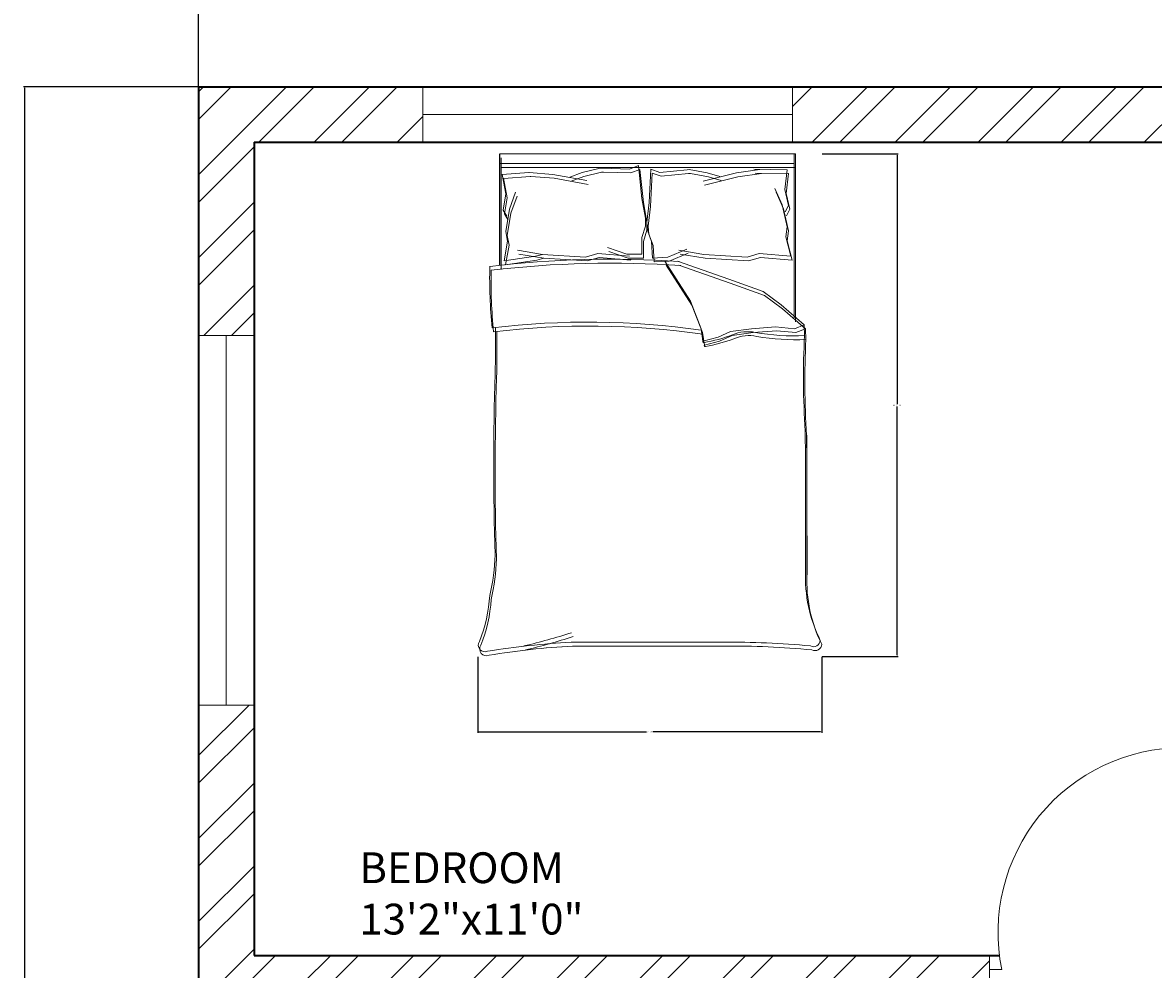
# Model space of a CAD drawing. Units: inches. Extents: x 1850 to 3445, y 1558 to 2756.
# Tile 3 of 13: x 2012 to 2195, y 2073 to 2227. Entities that reach past the tile are written whole.
import ezdxf

# ---------------------------------------------------------------- set-up
doc = ezdxf.new("R2010")
doc.units = ezdxf.units.IN
for name, color, linetype, lineweight in [('A-ANNO-DIMS', 2, 'Continuous', 18), ('A-AREA-IDEN', 7, 'Continuous', 18), ('A-DOOR', 3, 'Continuous', 18), ('A-FURN', 8, 'Continuous', 13), ('A-GLAZ', 4, 'Continuous', 18), ('A-WALL', 7, 'Continuous', 35), ('A-WALL-PATT', 252, 'Continuous', 13)]:
    doc.layers.add(name, color=color, linetype=linetype, lineweight=lineweight)
doc.styles.get("Standard").update_dxf_attribs({"font": 'arial.ttf'})
doc.dimstyles.get("Standard").update_dxf_attribs({"dimtxt": 0.18, "dimasz": 0.18, "dimexe": 0.18, "dimexo": 0.0625, "dimgap": 0.09, "dimtad": 0, "dimtih": 1, "dimtoh": 1, "dimdec": 4, "dimzin": 0, "dimdsep": 46, "dimtxsty": 'Standard', "dimcen": 0.09, "dimadec": 0, "dimazin": 0, "dimtfac": 1, "dimtdec": 4, "dimtofl": 0, "dimtmove": 0, "dimatfit": 3, "dimfxl": 1, "dimtolj": 1, "dimtzin": 0, "dimarcsym": 0})

# ---------------------------------------------------------------- blocks, each defined once
blk = doc.blocks.new('BED-PLAN')
for p, q in [((3.47, 63.33), (3.47, 81.44)), ((3.48, 63.33), (3.48, 81.44)), ((51.27, 81.44), (3.48, 81.44)), ((3.7, 62.69), (3.7, 80.8)), ((3.7, 62.69), (3.7, 80.8)), ((51.27, 81.44), (51.27, 54.83)), ((51.27, 81.44), (51.27, 54.83)), ((51.27, 81.44), (51.49, 81.44)), ((51.49, 81.44), (51.49, 80.8)), ((51.49, 80.8), (51.49, 54.19)), ((51.49, 80.8), (51.49, 54.19)), ((3.47, 79.91), (51.27, 79.91)), ((3.48, 79.91), (51.27, 79.91)), ((3.7, 79.27), (51.49, 79.27)), ((3.7, 79.27), (51.49, 79.27)), ((16.88, 78.42), (19.77, 79.14)), ((16.88, 78.42), (19.77, 79.14)), ((19.77, 79.14), (20.09, 79.14)), ((19.77, 79.14), (20.09, 79.14)), ((20.09, 79.14), (24.54, 78.99)), ((20.09, 79.14), (24.54, 78.99)), ((24.54, 78.99), (25.98, 79.57)), ((24.54, 78.99), (25.98, 79.57)), ((24.77, 78.36), (26.21, 78.93)), ((24.77, 78.36), (26.21, 78.93)), ((25.98, 79.57), (26.56, 74.22)), ((25.98, 79.57), (26.56, 74.22)), ((26.21, 78.93), (26.79, 73.58)), ((26.21, 78.93), (26.79, 73.58)), ((27.98, 78.95), (27.73, 73.58)), ((27.98, 78.95), (27.73, 73.58)), ((29.46, 78.46), (27.98, 78.95)), ((29.46, 78.46), (27.98, 78.95)), ((34.2, 78.91), (33.88, 78.89)), ((34.2, 78.91), (33.88, 78.89)), ((37.14, 78.36), (34.2, 78.91)), ((37.14, 78.36), (34.2, 78.91)), ((50.11, 78.89), (44.71, 78.98)), ((44.71, 78.98), (45.71, 78.9)), ((50.11, 78.89), (44.71, 78.98)), ((44.71, 78.98), (45.71, 78.9)), ((3.89, 78.13), (4.47, 74.95)), ((3.89, 78.13), (4.47, 74.95)), ((3.9, 78.11), (8.18, 78.43)), ((3.9, 78.11), (8.18, 78.43)), ((4.12, 77.49), (4.7, 74.31)), ((4.12, 77.49), (4.7, 74.31)), ((4.13, 77.47), (8.41, 77.8)), ((4.13, 77.47), (8.41, 77.8)), ((8.18, 78.43), (8.28, 78.42)), ((8.18, 78.43), (8.28, 78.42)), ((8.28, 78.42), (12.11, 78.13)), ((8.28, 78.42), (12.11, 78.13)), ((8.41, 77.8), (8.51, 77.78)), ((8.41, 77.8), (8.51, 77.78)), ((8.51, 77.78), (12.34, 77.49)), ((8.51, 77.78), (12.34, 77.49)), ((12.11, 78.13), (17.6, 77.11)), ((12.11, 78.13), (17.6, 77.11)), ((12.34, 77.49), (17.83, 76.48)), ((12.34, 77.49), (17.83, 76.48)), ((14.85, 77.69), (16.88, 78.42)), ((14.86, 77.69), (16.88, 78.42)), ((15.08, 77.05), (17.11, 77.78)), ((15.08, 77.05), (17.11, 77.78)), ((17.11, 77.78), (20, 78.5)), ((17.11, 77.78), (20, 78.5)), ((20, 78.5), (20.32, 78.5)), ((20, 78.5), (20.32, 78.5)), ((20.32, 78.5), (24.77, 78.36)), ((20.32, 78.5), (24.77, 78.36)), ((28.21, 78.31), (27.96, 72.94)), ((28.21, 78.31), (27.96, 72.94)), ((29.68, 77.83), (28.21, 78.31)), ((29.68, 77.83), (28.21, 78.31)), ((33.88, 78.89), (29.46, 78.46)), ((33.88, 78.89), (29.46, 78.46)), ((34.11, 78.25), (29.68, 77.83)), ((34.11, 78.25), (29.68, 77.83)), ((34.43, 78.27), (34.11, 78.25)), ((34.43, 78.27), (34.11, 78.25)), ((37.36, 77.73), (34.43, 78.27)), ((37.36, 77.73), (34.43, 78.27)), ((41.91, 78.37), (36.49, 77.02)), ((41.91, 78.37), (36.5, 77.02)), ((42.14, 77.73), (36.72, 76.38)), ((42.14, 77.73), (36.72, 76.38)), ((39.2, 77.77), (37.14, 78.36)), ((39.2, 77.77), (37.14, 78.36)), ((39.43, 77.13), (37.36, 77.73)), ((39.43, 77.13), (37.36, 77.73)), ((45.71, 78.9), (41.91, 78.37)), ((45.71, 78.9), (41.91, 78.37)), ((45.94, 78.26), (42.14, 77.73)), ((45.94, 78.26), (42.14, 77.73)), ((50.34, 78.25), (44.94, 78.34)), ((44.94, 78.34), (45.94, 78.26)), ((50.34, 78.25), (44.94, 78.34)), ((44.94, 78.34), (45.94, 78.26)), ((50.11, 78.89), (49.73, 75.68)), ((50.11, 78.89), (49.73, 75.68)), ((50.34, 78.25), (49.96, 75.04)), ((50.34, 78.25), (49.96, 75.04)), ((5.05, 72.49), (6.06, 75.24)), ((5.05, 72.49), (6.06, 75.24)), ((49.31, 73.19), (48.13, 75.86)), ((49.31, 73.19), (48.13, 75.86)), ((49.73, 75.68), (50.33, 73.1)), ((49.73, 75.68), (50.33, 73.1)), ((4.47, 74.95), (4.04, 72.34)), ((4.47, 74.95), (4.04, 72.34)), ((4.7, 74.31), (4.27, 71.7)), ((4.7, 74.31), (4.27, 71.7)), ((5.28, 71.85), (6.29, 74.6)), ((5.28, 71.85), (6.29, 74.6)), ((26.56, 74.22), (27.14, 71.04)), ((26.56, 74.22), (27.14, 71.04)), ((26.79, 73.58), (27.37, 70.4)), ((26.79, 73.58), (27.37, 70.4)), ((27.73, 73.58), (27.35, 70.37)), ((27.73, 73.58), (27.35, 70.37)), ((49.54, 72.55), (48.36, 75.23)), ((49.54, 72.55), (48.36, 75.23)), ((49.96, 75.04), (50.56, 72.47)), ((49.96, 75.04), (50.56, 72.47)), ((4.04, 72.34), (4.62, 71.33)), ((4.04, 72.34), (4.62, 71.33)), ((4.27, 71.7), (4.85, 70.69)), ((4.27, 71.7), (4.85, 70.69)), ((4.47, 68.87), (5.05, 72.49)), ((4.47, 68.87), (5.05, 72.49)), ((4.7, 68.23), (5.28, 71.85)), ((4.7, 68.23), (5.28, 71.85)), ((27.96, 72.94), (27.58, 69.73)), ((27.96, 72.94), (27.58, 69.73)), ((50.11, 69.61), (49.31, 73.19)), ((50.11, 69.61), (49.31, 73.19)), ((50.34, 68.98), (49.54, 72.55)), ((50.34, 68.98), (49.54, 72.55)), ((50.33, 73.1), (49.81, 72.06)), ((50.33, 73.1), (49.81, 72.06)), ((50.56, 72.47), (50.04, 71.42)), ((50.56, 72.47), (50.04, 71.42)), ((27.14, 69.74), (26.56, 67.86)), ((27.14, 69.74), (26.56, 67.86)), ((27.14, 71.04), (27.14, 69.74)), ((27.14, 71.04), (27.14, 69.74)), ((27.35, 70.37), (27.44, 69.07)), ((27.35, 70.37), (27.44, 69.07)), ((27.37, 70.4), (27.37, 69.1)), ((27.37, 70.4), (27.37, 69.1)), ((4.76, 67.28), (4.47, 68.87)), ((4.76, 67.28), (4.47, 68.87)), ((4.99, 66.64), (4.7, 68.23)), ((4.99, 66.64), (4.7, 68.23)), ((27.37, 69.1), (26.79, 67.22)), ((27.37, 69.1), (26.79, 67.22)), ((27.44, 69.07), (28.13, 67.23)), ((27.44, 69.07), (28.13, 67.23)), ((27.58, 69.73), (27.66, 68.43)), ((27.58, 69.73), (27.66, 68.43)), ((27.66, 68.43), (28.36, 66.59)), ((27.66, 68.43), (28.36, 66.59)), ((49.92, 68.01), (50.11, 69.61)), ((49.92, 68.01), (50.11, 69.61)), ((50.7, 64.87), (49.92, 68.01)), ((50.7, 64.87), (49.92, 68.01)), ((50.15, 67.37), (50.34, 68.98)), ((50.15, 67.37), (50.34, 68.98)), ((4.18, 64.1), (4.76, 67.28)), ((4.18, 64.1), (4.76, 67.28)), ((4.41, 63.46), (4.99, 66.64)), ((4.41, 63.46), (4.99, 66.64)), ((24.1, 65.18), (20.96, 66.27)), ((24.1, 65.18), (20.96, 66.27)), ((26.56, 67.86), (26.56, 65.18)), ((26.56, 67.86), (26.56, 65.18)), ((26.79, 67.22), (26.79, 64.54)), ((26.79, 67.22), (26.79, 64.54)), ((28.13, 67.23), (28.3, 64.55)), ((28.13, 67.23), (28.3, 64.55)), ((28.36, 66.59), (28.53, 63.91)), ((28.36, 66.59), (28.53, 63.91)), ((50.93, 64.23), (50.15, 67.37)), ((50.93, 64.23), (50.15, 67.37)), ((9.28, 64.83), (4.18, 64.1)), ((9.28, 64.83), (4.18, 64.1)), ((6.38, 65.81), (10.41, 65.15)), ((6.38, 65.81), (10.41, 65.15)), ((6.61, 65.18), (10.64, 64.51)), ((6.61, 65.18), (10.64, 64.51)), ((10.41, 65.15), (9.28, 64.83)), ((10.41, 65.15), (9.28, 64.83)), ((10.64, 64.51), (9.51, 64.19)), ((10.64, 64.51), (9.51, 64.19)), ((10.41, 65.15), (17.42, 64.72)), ((10.41, 65.15), (17.42, 64.72)), ((10.64, 64.51), (17.65, 64.08)), ((10.64, 64.51), (17.65, 64.08)), ((17.42, 64.72), (19.38, 65.27)), ((17.42, 64.72), (19.38, 65.27)), ((17.65, 64.08), (19.61, 64.63)), ((17.65, 64.08), (19.61, 64.63)), ((19.38, 65.27), (24.52, 64.87)), ((19.38, 65.27), (24.52, 64.87)), ((19.61, 64.63), (24.74, 64.23)), ((19.61, 64.63), (24.74, 64.23)), ((24.33, 64.54), (21.19, 65.63)), ((24.33, 64.54), (21.19, 65.63)), ((26.56, 65.18), (24.1, 65.18)), ((26.56, 65.18), (24.1, 65.18)), ((26.79, 64.54), (24.33, 64.54)), ((26.79, 64.54), (24.33, 64.54)), ((28.3, 64.55), (30.75, 64.7)), ((28.3, 64.55), (30.75, 64.7)), ((30.75, 64.7), (33.82, 65.99)), ((30.75, 64.7), (33.82, 65.99)), ((30.98, 64.06), (34.05, 65.35)), ((30.98, 64.06), (34.05, 65.35)), ((32.56, 65.81), (36.6, 65.15)), ((32.56, 65.81), (36.6, 65.15)), ((32.79, 65.18), (36.82, 64.51)), ((32.79, 65.18), (36.82, 64.51)), ((36.6, 65.15), (43.61, 64.72)), ((36.6, 65.15), (43.61, 64.72)), ((36.82, 64.51), (43.83, 64.08)), ((36.82, 64.51), (43.83, 64.08)), ((43.61, 64.72), (45.57, 65.27)), ((43.61, 64.72), (45.57, 65.27)), ((43.83, 64.08), (45.79, 64.63)), ((43.83, 64.08), (45.79, 64.63)), ((45.57, 65.27), (50.7, 64.87)), ((45.57, 65.27), (50.7, 64.87)), ((45.79, 64.63), (50.93, 64.23)), ((45.79, 64.63), (50.93, 64.23)), ((9.51, 64.19), (4.41, 63.46)), ((9.51, 64.19), (4.41, 63.46)), ((28.53, 63.91), (30.98, 64.06)), ((28.53, 63.91), (30.98, 64.06)), ((30.26, 64.06), (34.45, 57.57)), ((30.26, 64.06), (34.45, 57.57)), ((30.49, 63.42), (34.68, 56.93)), ((30.49, 63.42), (34.68, 56.93)), ((40.64, 61.13), (32.31, 64.06)), ((40.64, 61.13), (32.31, 64.06)), ((40.87, 60.49), (32.53, 63.42)), ((40.87, 60.49), (32.53, 63.42)), ((46.22, 59.11), (40.64, 61.13)), ((46.22, 59.11), (40.64, 61.13)), ((46.45, 58.48), (40.87, 60.49)), ((46.45, 58.48), (40.87, 60.49)), ((49.16, 56.95), (46.22, 59.11)), ((49.16, 56.95), (46.22, 59.11)), ((34.45, 57.57), (36.15, 53.08)), ((34.45, 57.57), (36.15, 53.08)), ((34.68, 56.93), (36.38, 52.44)), ((34.68, 56.93), (36.38, 52.44)), ((49.39, 56.31), (46.45, 58.48)), ((49.39, 56.31), (46.45, 58.48)), ((52.87, 53.7), (49.16, 56.95)), ((52.87, 53.7), (49.16, 56.95)), ((53.1, 53.06), (49.39, 56.31)), ((53.1, 53.06), (49.39, 56.31)), ((44.36, 53.08), (48.23, 53.39)), ((44.36, 53.08), (48.23, 53.39)), ((48.23, 53.39), (51.33, 53.08)), ((48.23, 53.39), (51.33, 53.08)), ((51.33, 53.08), (52.87, 53.7)), ((51.33, 53.08), (52.87, 53.7)), ((52.95, 51.95), (52.87, 53.7, 3.87)), ((52.95, 51.95), (52.87, 53.7, 3.87)), ((36.15, 53.08), (36.46, 51.07)), ((36.15, 53.08), (36.46, 51.07)), ((36.38, 52.44), (36.69, 50.43)), ((36.38, 52.44), (36.69, 50.43)), ((36.46, 51.07), (38.94, 51.69)), ((36.46, 51.07), (38.94, 51.69)), ((38.94, 51.69), (40.95, 52.61)), ((38.94, 51.69), (40.95, 52.61)), ((39.17, 51.05), (41.18, 51.97)), ((39.17, 51.05), (41.18, 51.97)), ((40.95, 52.61), (44.36, 53.08)), ((40.95, 52.61), (44.36, 53.08)), ((41.18, 51.97), (44.59, 52.44)), ((41.18, 51.97), (44.59, 52.44)), ((44.59, 52.44), (48.46, 52.75)), ((44.59, 52.44), (48.46, 52.75)), ((48.46, 52.75), (51.56, 52.44)), ((48.46, 52.75), (51.56, 52.44)), ((51.56, 52.44), (53.1, 53.06)), ((51.56, 52.44), (53.1, 53.06)), ((53.18, 51.31), (53.1, 53.06, 3.87)), ((53.18, 51.31), (53.1, 53.06, 3.87)), ((36.69, 50.43), (39.17, 51.05)), ((36.69, 50.43), (39.17, 51.05)), ((15.06, 2.2), (39.68, 2.2)), ((15.06, 2.2), (39.68, 2.2)), ((15.29, 1.56), (39.91, 1.56)), ((15.29, 1.56), (39.91, 1.56))]:
    blk.add_line(p, q)
for centre, radius, start, end in [((21.36, -100.61), 164.97, 86.0865, 96.7821), ((21.36, -100.61), 164.97, 86.0865, 96.7821), ((85.16, 61.35), 83.31, 178.7218, 185.604), ((85.16, 61.35), 83.31, 178.7218, 185.604), ((85.39, 60.71), 83.31, 178.7218, 185.604), ((85.39, 60.71), 83.31, 178.7218, 185.604), ((21.59, -101.25), 164.97, 86.0865, 96.7821), ((21.59, -101.25), 164.97, 86.0865, 96.7821), ((17.76, -74.87), 129.02, 81.7845, 96.9006), ((17.76, -74.87), 129.02, 81.7845, 96.9006), ((17.98, -75.51), 129.02, 81.7845, 96.9006), ((17.98, -75.51), 129.02, 81.7845, 96.9006), ((-167.31, 50.27), 170.11, 358.4762, 1.0082), ((-167.31, 50.27), 170.11, 358.4762, 1.0082), ((-167.08, 49.63), 170.11, 358.4762, 1.0082), ((-167.08, 49.63), 170.11, 358.4762, 1.0082), ((31.15, 79.96), 29.65, 280.6617, 289.8806), ((31.15, 79.96), 29.65, 280.6617, 289.8806), ((31.38, 79.32), 29.65, 280.6617, 289.8806), ((31.38, 79.32), 29.65, 280.6617, 289.8806), ((43.74, 46.38), 6.22, 78.6608, 113.7384), ((43.74, 46.38), 6.22, 78.6608, 113.7384), ((43.97, 45.74), 6.22, 78.6608, 113.7384), ((43.97, 45.74), 6.22, 78.6608, 113.7384), ((51.33, 88.1), 36.18, 259.8763, 272.5657), ((51.33, 88.1), 36.18, 259.8763, 272.5657), ((51.56, 87.46), 36.18, 259.8763, 272.5657), ((51.56, 87.46), 36.18, 259.8763, 272.5657), ((182.27, 45.13), 129.5, 176.9791, 183.8365), ((182.27, 45.13), 129.5, 176.9791, 183.8365), ((36.64, 51), 0.185, 160.2464, 271.1377), ((36.64, 51), 0.185, 160.2464, 271.1377), ((36.86, 50.36), 0.185, 160.2464, 271.1377), ((36.86, 50.36), 0.185, 160.2464, 271.1377), ((182.49, 44.49), 129.5, 176.9791, 183.8365), ((182.49, 44.49), 129.5, 176.9791, 183.8365), ((484.82, 30.83), 482.31, 178.2277, 181.7185), ((484.82, 30.83), 482.31, 178.2277, 181.7185), ((485.05, 30.19), 482.31, 178.2277, 181.7185), ((485.05, 30.19), 482.31, 178.2277, 181.7185), ((-4508.74, 13.62), 4561.86, 0.00217, 0.28689), ((-4508.74, 13.62), 4561.86, 0.00217, 0.28689), ((-4508.51, 12.98), 4561.86, 0.00217, 0.28689), ((-4508.52, 12.98), 4561.86, 0.00217, 0.28689), ((-26.9, 16.93), 29.63, 346.0648, 358.9113), ((-26.9, 16.93), 29.63, 346.0648, 358.9113), ((-26.67, 16.29), 29.63, 346.0648, 358.9113), ((-26.67, 16.29), 29.63, 346.0648, 358.9113), ((76.16, 12.78), 23.07, 177.4714, 206.4681), ((76.16, 12.78), 23.07, 177.4714, 206.4681), ((76.39, 12.14), 23.07, 177.4714, 206.4681), ((76.39, 12.14), 23.07, 177.4714, 206.4681), ((-21.66, 11.17), 23.56, 337.9751, 356.652), ((-21.66, 11.17), 23.56, 337.9751, 356.652), ((-21.43, 10.53), 23.56, 337.9751, 356.652), ((-21.43, 10.53), 23.56, 337.9751, 356.652), ((-17.22, 105.16), 106.46, 283.3832, 287.7053), ((-17.22, 105.16), 106.46, 283.3832, 287.7053), ((1.09, 1.73), 1.09, 146.1736, 293.4781), ((1.09, 1.73), 1.09, 146.1736, 293.4781), ((21.43, -119.39), 121.76, 92.9958, 99.4091), ((21.43, -119.39), 121.76, 92.9958, 99.4091), ((-16.99, 104.52), 106.46, 283.3832, 287.7053), ((-16.99, 104.52), 106.46, 283.3832, 287.7053), ((41.15, -130.83), 133.04, 84.4998, 90.6351), ((41.15, -130.83), 133.04, 84.4998, 90.6351), ((54.41, 2.57), 1.1, 242.6588, 356.02), ((54.41, 2.57), 1.1, 242.6588, 356.02), ((54.64, 1.93), 1.1, 242.6588, 356.02), ((54.64, 1.93), 1.1, 242.6588, 356.02), ((1.32, 1.09), 1.09, 146.1736, 293.4781), ((1.32, 1.09), 1.09, 146.1736, 293.4781), ((21.66, -120.03), 121.76, 92.9958, 99.4091), ((21.65, -120.03), 121.76, 92.9958, 99.4091), ((41.38, -131.47), 133.04, 84.4998, 90.6351), ((41.38, -131.47), 133.04, 84.4998, 90.6351)]:
    blk.add_arc(centre, radius, start, end)
blk = doc.blocks.new('WIN-60-W9')
for p, q in [((0, 9), (0, 0)), ((60, 4.5), (60, 9)), ((60, 9), (60, 0)), ((0, 0), (0, 4.5)), ((0, 4.5), (60, 4.5))]:
    blk.add_line(p, q)
blk = doc.blocks.new('WIN-60-W9-ALT')
for p, q in [((9, 60), (0, 60)), ((0, 60), (4.5, 60)), ((4.5, 60), (4.5, 0)), ((4.5, 0), (0, 0)), ((0, 0), (9, 0))]:
    blk.add_line(p, q)
blk = doc.blocks.new('DOOR-BED-GROUND')
for p, q in [((31.38, 2.25), (31.38, 38.25)), ((0, 4.5), (0, 0)), ((33.38, 4.5), (33.38, 0)), ((0, 0), (0, 2.25)), ((0, 2.25), (2, 2.25)), ((33.38, 2.25), (31.38, 2.25)), ((33.38, 0), (33.38, 2.25))]:
    blk.add_line(p, q)
blk.add_arc((31.38, 8.26), 29.99, 90, 191.5706)
blk = doc.blocks.new('*D50')
at = {"layer": 'A-ANNO-DIMS', "color": 0, "lineweight": -2, "transparency": 16777216}
for p, q in [((2141.46, 2205.28), (2153.81, 2205.28)), ((2153.63, 2205.1), (2153.63, 2164.69)), ((2153.63, 2123.91), (2153.63, 2164.32)), ((2141.46, 2123.73), (2153.81, 2123.73))]:
    blk.add_line(p, q, dxfattribs=at)
at = {"layer": 'A-ANNO-DIMS', "color": 0, "transparency": 16777216}
for points in [[(2153.6, 2205.1), (2153.66, 2205.1), (2153.63, 2205.28)], [(2153.6, 2123.91), (2153.66, 2123.91), (2153.63, 2123.73)]]:
    blk.add_solid(points, dxfattribs=at)
at = {"layer": 'Defpoints', "color": 0, "transparency": 16777216}
for p in [(2141.39, 2205.28), (2153.63, 2205.28), (2141.39, 2123.73)]:
    blk.add_point(p, dxfattribs=at)
at = {"layer": 'A-ANNO-DIMS', "color": 0, "transparency": 16777216, "insert": (2153.63, 2164.51), "char_height": 0.18, "attachment_point": 5}
blk.add_mtext('\\A1;BED 82 TYP.', dxfattribs=at)
blk = doc.blocks.new('*D51')
at = {"layer": 'A-ANNO-DIMS', "color": 0, "lineweight": -2, "transparency": 16777216}
for p, q in [((2085.57, 2123.67), (2085.57, 2111.32)), ((2141.39, 2123.67), (2141.39, 2111.32)), ((2085.75, 2111.5), (2112.95, 2111.5)), ((2141.21, 2111.5), (2114.01, 2111.5))]:
    blk.add_line(p, q, dxfattribs=at)
at = {"layer": 'A-ANNO-DIMS', "color": 0, "transparency": 16777216}
for points in [[(2085.75, 2111.53), (2085.75, 2111.47), (2085.57, 2111.5)], [(2141.21, 2111.53), (2141.21, 2111.47), (2141.39, 2111.5)]]:
    blk.add_solid(points, dxfattribs=at)
at = {"layer": 'Defpoints', "color": 0, "transparency": 16777216}
for p in [(2085.57, 2123.73), (2141.39, 2123.73), (2141.39, 2111.5)]:
    blk.add_point(p, dxfattribs=at)
at = {"layer": 'A-ANNO-DIMS', "color": 0, "transparency": 16777216, "insert": (2113.48, 2111.5), "char_height": 0.18, "attachment_point": 5}
blk.add_mtext('\\A1;56 TYP.', dxfattribs=at)
blk = doc.blocks.new('*D80')
at = {"layer": 'A-ANNO-DIMS', "color": 0, "lineweight": -2, "transparency": 16777216}
for p, q in [((2040.27, 2216.25), (2040.27, 2244.61)), ((2040.45, 2244.43), (2162.48, 2244.43)), ((2285.09, 2244.43), (2163.06, 2244.43)), ((2285.27, 2216.25), (2285.27, 2244.61))]:
    blk.add_line(p, q, dxfattribs=at)
at = {"layer": 'A-ANNO-DIMS', "color": 0, "transparency": 16777216}
for points in [[(2040.45, 2244.46), (2040.45, 2244.4), (2040.27, 2244.43)], [(2285.09, 2244.46), (2285.09, 2244.4), (2285.27, 2244.43)]]:
    blk.add_solid(points, dxfattribs=at)
at = {"layer": 'Defpoints', "color": 0, "transparency": 16777216}
for p in [(2285.27, 2244.43), (2040.27, 2216.18), (2285.27, 2216.18)]:
    blk.add_point(p, dxfattribs=at)
at = {"layer": 'A-ANNO-DIMS', "color": 0, "transparency": 16777216, "insert": (2162.77, 2244.43), "char_height": 0.18, "attachment_point": 5}
blk.add_mtext('\\A1;245', dxfattribs=at)
blk = doc.blocks.new('*D81')
at = {"layer": 'A-ANNO-DIMS', "color": 0, "lineweight": -2, "transparency": 16777216}
for p, q in [((2040.21, 2216.18), (2011.84, 2216.18)), ((2012.02, 2216), (2012.02, 1981.12)), ((2012.02, 1745.86), (2012.02, 1980.75)), ((2040.21, 1745.68), (2011.84, 1745.68))]:
    blk.add_line(p, q, dxfattribs=at)
at = {"layer": 'A-ANNO-DIMS', "color": 0, "transparency": 16777216}
for points in [[(2011.99, 2216), (2012.05, 2216), (2012.02, 2216.18)], [(2011.99, 1745.86), (2012.05, 1745.86), (2012.02, 1745.68)]]:
    blk.add_solid(points, dxfattribs=at)
at = {"layer": 'Defpoints', "color": 0, "transparency": 16777216}
for p in [(2012.02, 2216.18), (2040.27, 2216.18), (2040.27, 1745.68)]:
    blk.add_point(p, dxfattribs=at)
at = {"layer": 'A-ANNO-DIMS', "color": 0, "transparency": 16777216, "insert": (2012.02, 1980.93), "char_height": 0.18, "attachment_point": 5}
blk.add_mtext('\\A1;470.5', dxfattribs=at)

msp = doc.modelspace()

# ---------------------------------------------------------------- hatches: boundary and pattern name
at = {"layer": 'A-WALL-PATT'}
h = msp.add_hatch(dxfattribs=at)
h.set_pattern_fill('ANSI32', color=256)
h.paths.add_polyline_path([(2519.5556, 1907.3936), (2523.9987, 1907.3936), (2523.9987, 1916.3936), (2519.5556, 1916.3936), (2515.0556, 1916.3936), (2510.5556, 1916.3936), (2510.5556, 1907.3936), (2515.0556, 1907.3936), (2515.0556, 1742.1843), (2515.0556, 1737.6843), (2596.0556, 1737.6843), (2596.0556, 1976.4962), (2591.5556, 1976.4962), (2591.5556, 1916.3936), (2561.2666, 1916.3936), (2561.2666, 1907.3936), (2591.5556, 1907.3936), (2591.5556, 1746.6843), (2519.5556, 1746.6843)])
h.paths.add_polyline_path([(2076.6481, 2211.6843), (2076.6481, 2216.1843), (2040.2715, 2216.1843), (2040.2715, 2175.83), (2044.7715, 2175.83), (2049.2715, 2175.83), (2049.2715, 2207.1843), (2076.6481, 2207.1843)])
h.paths.add_polyline_path([(2211.7715, 2216.1843), (2136.6481, 2216.1843), (2136.6481, 2207.1843), (2211.7715, 2207.1843)])
h.paths.add_polyline_path([(2285.2715, 2154.1843), (2250.6169, 2154.1843), (2250.6169, 2149.6843), (2280.7715, 2149.6843), (2280.7715, 2075.1843), (2236.3632, 2075.1843), (2236.3632, 2070.6843), (2285.2715, 2070.6843)])
h.paths.add_polyline_path([(2228.3485, 2154.1843), (2207.2715, 2154.1843), (2207.2715, 2075.1843), (2201.9819, 2075.1843), (2201.9819, 2070.6843), (2215.4663, 2070.6843), (2215.4663, 2072.9343), (2215.4663, 2075.1843), (2211.7715, 2075.1843), (2211.7715, 2149.6843), (2228.3485, 2149.6843)])
h.paths.add_polyline_path([(2049.2715, 2115.83), (2040.2715, 2115.83), (2040.2715, 2042.8465), (2049.2715, 2042.8465), (2049.2715, 2070.6843), (2168.6057, 2070.6843), (2168.6057, 2072.9343), (2168.6057, 2075.1843), (2049.2715, 2075.1843)])
h.paths.add_polyline_path([(2049.2715, 1982.8465), (2040.2715, 1982.8465), (2040.2715, 1910.2175), (2060.9481, 1910.2175), (2060.9481, 1914.7175), (2060.9481, 1919.2175), (2049.2715, 1919.2175)])
h.paths.add_polyline_path([(2132.4938, 1919.2175), (2108.9481, 1919.2175), (2108.9481, 1910.2175), (2132.4938, 1910.2175), (2132.4938, 1914.6749)])
h.paths.add_polyline_path([(2178.7715, 1938.6843), (2169.7715, 1938.6843), (2169.7715, 1919.2175), (2163.687, 1919.2175), (2163.687, 1910.2175), (2169.7715, 1910.2175), (2169.7715, 1854.6843), (2169.7715, 1845.6843), (2196.1287, 1845.6843), (2196.1287, 1850.1843), (2196.1287, 1854.6843), (2178.7715, 1854.6843)])
h.paths.add_polyline_path([(2049.2715, 1910.2175), (2040.2715, 1910.2175), (2040.2715, 1745.6843), (2049.2715, 1745.6843)])
h.paths.add_polyline_path([(2146.8861, 1766.7204), (2159.0894, 1766.7204), (2159.0894, 1777.0239), (2146.8861, 1777.0239)], flags=9)
h.paths.add_polyline_path([(2183.4664, 1798.4016), (2226.7338, 1798.4016), (2226.7338, 1817.0589), (2183.4664, 1817.0589)], flags=9)
h.paths.add_polyline_path([(2070.863, 1867.537), (2109.9796, 1867.537), (2109.9796, 1886.1943), (2070.863, 1886.1943)], flags=9)

# ---------------------------------------------------------------- linework, layer by layer
at = {"layer": 'A-WALL'}
for p, q in [((2040.2715, 2216.1843), (2285.2715, 2216.1843)), ((2040.2715, 2216.1843), (2040.2715, 1745.6843)), ((2049.2715, 2207.1843), (2211.7715, 2207.1843)), ((2049.2715, 2207.1843), (2049.2715, 2075.1843)), ((2049.2715, 2075.1843), (2170.2335, 2075.1843))]:
    msp.add_line(p, q, dxfattribs=at)

# ---------------------------------------------------------------- block references
at = {"layer": 'A-DOOR'}
msp.add_blockref('DOOR-BED-GROUND', (2168.606, 2070.684), dxfattribs=at)
at = {"layer": 'A-FURN'}
msp.add_blockref('BED-PLAN', (2085.655, 2123.837), dxfattribs=at)
at = {"layer": 'A-GLAZ'}
for name, p in [('WIN-60-W9', (2076.648, 2207.184)), ('WIN-60-W9-ALT', (2040.271, 2115.83))]:
    msp.add_blockref(name, p, dxfattribs=at)

# ---------------------------------------------------------------- texts
at = {"layer": 'A-AREA-IDEN', "insert": (2066.3578, 2091.9299), "char_height": 5, "attachment_point": 1}
msp.add_mtext_dynamic_manual_height_columns('BEDROOM\\P13\'2"x11\'0"', width=133.624147, gutter_width=12.5, heights=[0], dxfattribs=at)

# ---------------------------------------------------------------- dimensions: what is measured, and where the dimension line sits
at = {"layer": 'A-ANNO-DIMS'}
dim = msp.add_linear_dim(base=(2285.2715, 2244.4343), p1=(2040.2715, 2216.1843), p2=(2285.2715, 2216.1843), dimstyle='Standard', override={"dimdec": 0, "dimlfac": 1, "dimrnd": 0, "dimzin": 0, "dimdsep": 46, "dimlunit": 2}, dxfattribs=at)
dim.commit()
dim.dimension.update_dxf_attribs({"geometry": '*D80', "text_midpoint": (2162.7715, 2244.4343)})
dim = msp.add_linear_dim(base=(2012.0215, 2216.1843), p1=(2040.2715, 1745.6843), p2=(2040.2715, 2216.1843), angle=90, dimstyle='Standard', override={"dimdec": 1, "dimlfac": 1, "dimrnd": 0, "dimzin": 0, "dimdsep": 46, "dimlunit": 2}, dxfattribs=at)
dim.commit()
dim.dimension.update_dxf_attribs({"geometry": '*D81', "text_midpoint": (2012.0215, 1980.9343)})
dim = msp.add_linear_dim(base=(2153.6255, 2205.2802), p1=(2141.3932, 2123.7316), p2=(2141.3932, 2205.2802), angle=90, text='BED <> TYP.', dimstyle='Standard', override={"dimdec": 0, "dimlfac": 1, "dimrnd": 0, "dimzin": 0, "dimdsep": 46, "dimlunit": 2}, dxfattribs=at)
dim.commit()
dim.dimension.update_dxf_attribs({"geometry": '*D50', "text_midpoint": (2153.6255, 2164.5059)})
dim = msp.add_linear_dim(base=(2141.3932, 2111.4993), p1=(2085.5686, 2123.7316), p2=(2141.3932, 2123.7316), text='<> TYP.', dimstyle='Standard', override={"dimdec": 0, "dimlfac": 1, "dimrnd": 0, "dimzin": 0, "dimdsep": 46, "dimlunit": 2}, dxfattribs=at)
dim.commit()
dim.dimension.update_dxf_attribs({"geometry": '*D51', "text_midpoint": (2113.4809, 2111.4993)})

doc.saveas('drawing.dxf')
